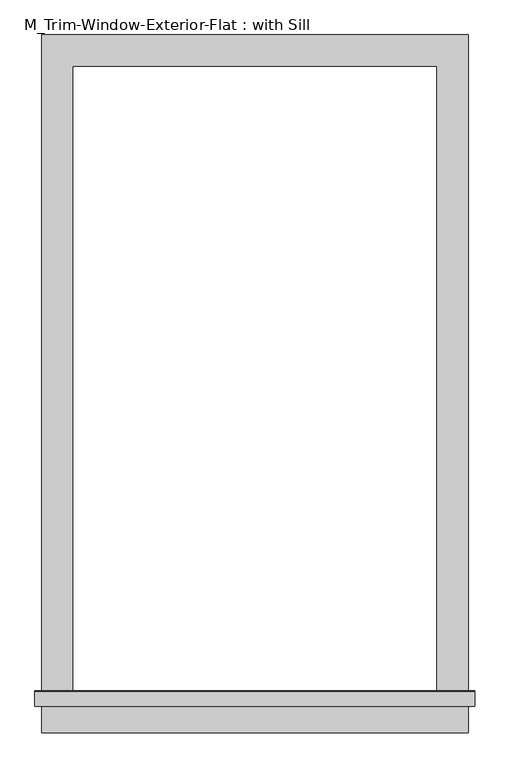
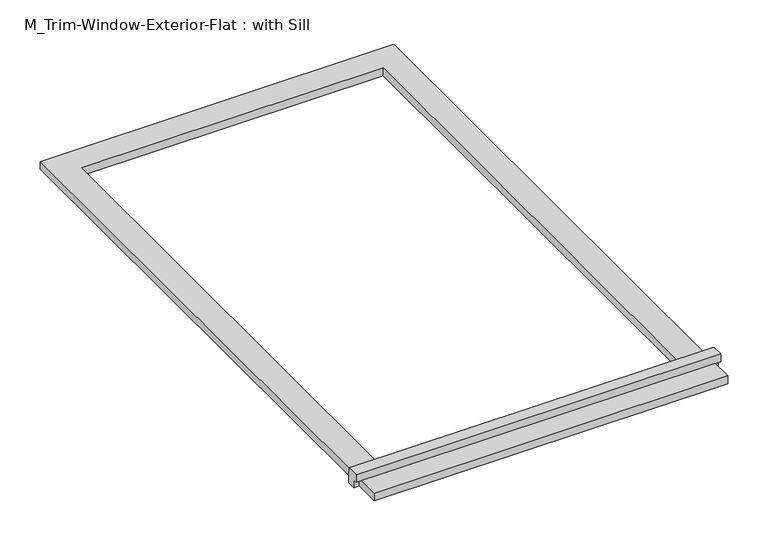
"""IFC4 building model written with IfcOpenShell, lengths in millimetres: proxy geometry, M_Trim-Window-Exterior-Flat : with Sill."""

from ifc_helpers import new_model, si_unit, frame, origin, origin_with_axes, place, context, project, spatial, polyline, outline, extrude, source, transform, mapped, element, save


def m_trim_window_exterior_flat_with_sill_7a42a2ef(model_context):
    return source(origin(), model_context, "Body", "SweptSolid", [
        extrude(outline(polyline([(410.0, -1220.4323709), (410.0, -1280.4323709), (-410.0, -1280.4323709), (-410.0, -1220.4323709), (410.0, -1220.4323709)])), origin_with_axes(), (0.0, 0.0, 1.0), 19.05),
        extrude(outline(polyline([(-1230.0, 38.1), (-1202.4580645, 38.1), (-1200.0, 19.05), (-1200.0, 0.0), (-1220.4323709, 0.0), (-1220.4323709, 19.05), (-1230.0, 19.05), (-1230.0, 38.1)])), frame((-422.7, 0.0, 0.0), z_axis=(1.0, 0.0, 0.0), x_axis=(0.0, 1.0, 0.0)), (0.0, 0.0, 1.0), 845.4),
        extrude(outline(polyline([(-410.0, 60.0), (410.0, 60.0), (410.0, -1200.0), (350.0, -1200.0), (350.0, 0.0), (-350.0, 0.0), (-350.0, -1200.0), (-410.0, -1200.0), (-410.0, 60.0)])), origin_with_axes(), (0.0, 0.0, 1.0), 19.05),
    ])


if __name__ == "__main__":
    model = new_model("IFC4")
    model_context = context("Model", 3, world=origin())
    ifc_project = project(units=[si_unit("LENGTHUNIT", "METRE", prefix="MILLI")], contexts=[model_context])
    site = spatial("IfcSite", under=ifc_project)
    building = spatial("IfcBuilding", under=site)
    placement = place(None, origin())
    m_trim_window_exterior_flat_with_sill_shape = m_trim_window_exterior_flat_with_sill_7a42a2ef(model_context)
    element("IfcBuildingElementProxy", 1, Name="M_Trim-Window-Exterior-Flat : with Sill", ObjectType="M_Trim-Window-Exterior-Flat : with Sill", at=placement, inside=building, context=model_context, shape_type="MappedRepresentation", body=[
        mapped(m_trim_window_exterior_flat_with_sill_shape, transform((0.0, 0.0, 0.0), x_axis=(1.0, 0.0, 0.0), y_axis=(0.0, 1.0, 0.0), z_axis=(0.0, 0.0, 1.0))),
    ])
    save(model, "model.ifc")

# Revit data of these elements
# Type "M_Trim-Window-Exterior-Flat : with Sill"
#   Trim Width = 0.06 m
#   Trim Thickness_Picture Frame = 0.03 m
#   Trim Thickness_with Sill = 0.01905 m
#   Sill Thickness = 0.03 m
#   Opening Width [instance default] = 0.6 m
#   Opening Height [instance default] = 0.9 m
#   Default Elevation = 1.2 m
#   Sill = yes
#   Picture Frame = no
#   Trim Material [instance default] = none
# Element 1 (IfcBuildingElementProxy, "M_Trim-Window-Exterior-Flat : with Sill")
#   Opening Width = 0.7 m
#   Opening Height = 1.2 m
#   Trim Material = Clad - White
#   Materials on its faces: "Clad - White"
# Materials
#   "Clad - White": class "Wood", colour RGB 242 242 238, transparency 0, Cost = 0
